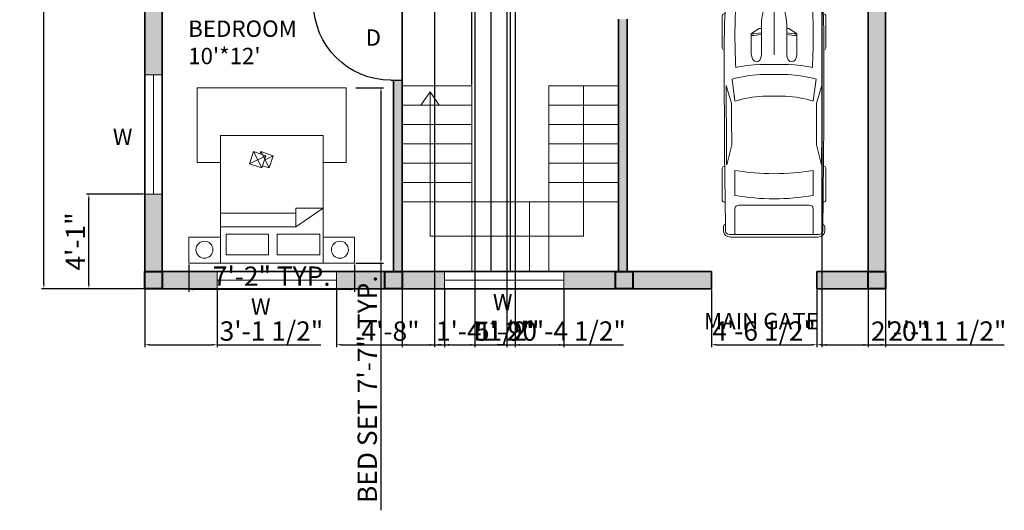
# Model space of a CAD drawing. Units: inches. Extents: x 1801 to 2333, y 2020 to 2714.
# Tile 1 of 4: x 1801 to 2311, y 2020 to 2274. Entities that reach past the tile are written whole.
import ezdxf

# ---------------------------------------------------------------- set-up
doc = ezdxf.new("R2010")
doc.units = ezdxf.units.IN
for name, color, linetype, lineweight in [('A-ANNO-DIMS', 2, 'Continuous', 18), ('A-ANNO-TEXT', 200, 'Continuous', 18), ('A-AREA-IDEN', 200, 'Continuous', 25), ('A-COLS', 7, 'Continuous', 40), ('A-COLS-PATT', 250, 'Continuous', 13), ('A-DOOR', 4, 'Continuous', 25), ('A-FLOR-STRS', 7, 'Continuous', 18), ('A-FURN', 8, 'Continuous', 18), ('A-SITE-VEHI', 8, 'Continuous', 13), ('A-WALL-PATT', 252, 'Continuous', 13), ('WALL', 150, 'Continuous', 35), ('WINDOW', 130, 'Continuous', 18)]:
    doc.layers.add(name, color=color, linetype=linetype, lineweight=lineweight)
doc.styles.get("Standard").update_dxf_attribs({"font": 'arial.ttf'})
doc.dimstyles.new('ISO-25', dxfattribs={"dimtxt": 10, "dimasz": 2.5, "dimexe": 1.25, "dimexo": 0.625, "dimtad": 1, "dimdec": 0, "dimlunit": 4, "dimtxsty": 'Standard', "dimcen": 2.5, "dimadec": 0, "dimazin": 0, "dimtfac": 1, "dimtdec": 0, "dimtmove": 0, "dimatfit": 3, "dimfxl": 1, "dimarcsym": 0})

# ---------------------------------------------------------------- blocks, each defined once
blk = doc.blocks.new('*U2')
for p, q in [((0, 0), (0, -6)), ((40, 0), (40, -6))]:
    blk.add_line(p, q)
blk.add_lwpolyline([(0, 0), (0, 40), (1.75, 40), (1.75, 0)], close=True)
blk.add_arc((0, 0), 40, 0, 90)
blk = doc.blocks.new('*U6')
for p, q in [((21.1, 37.41), (21.1, 36.83)), ((46.55, 38.89), (22.35, 38.89)), ((47.8, 37.39), (47.8, 37.41)), ((135.45, 37.07), (135.45, 37.41)), ((136.7, 38.89), (160.9, 38.89)), ((162.15, 37.41), (162.15, 36.77)), ((70.03, 31.54), (86.41, 29.35)), ((87.99, 31.87), (74.76, 35.92)), ((134.31, 35.6), (119.29, 31.78)), ((186.47, -33.5), (186.47, 33.5)), ((188.4, -32.76), (188.4, 32.76)), ((138.42, 29.35), (157.25, 29.35)), ((164.52, 26.39), (164.52, -26.39)), ((186.47, 29.35), (167.01, 29.35)), ((32.27, 11.63), (36.13, 17.17)), ((36.13, 17.17), (50.94, 17.17)), ((29.77, 9.51), (51.68, 9.51)), ((32.12, 9.51), (32.12, 11.15)), ((58.92, -10.77), (58.92, 10.77)), ((66.55, -10.53), (66.55, 10.53)), ((82.74, 8.5), (82.74, -8.5)), ((186.47, -10.53), (186.47, 10.53)), ((3.27, 6.13), (0.1, 0.41)), ((0, 0), (51.68, 0)), ((0.1, -0.41), (3.27, -6.13)), ((29.77, -9.51), (51.68, -9.51)), ((32.12, -9.51), (32.12, -11.15)), ((32.27, -11.63), (36.13, -17.17)), ((36.13, -17.17), (50.94, -17.17)), ((86.41, -29.35), (70.03, -31.54)), ((157.25, -29.35), (138.42, -29.35)), ((167.01, -29.35), (186.47, -29.35)), ((21.1, -37.41), (21.1, -36.83)), ((87.99, -31.87), (74.76, -35.92)), ((134.31, -35.6), (119.29, -31.78)), ((162.15, -37.41), (162.15, -36.77)), ((46.55, -38.89), (22.35, -38.89)), ((47.8, -37.39), (47.8, -37.41)), ((135.45, -37.07), (135.45, -37.41)), ((136.7, -38.89), (160.9, -38.89))]:
    blk.add_line(p, q)
for centre, major_axis, ratio, start_param, end_param in [((41.19, -490.86), (0, 528.23), 0.842304, 0.00281, 0.075598), ((22.35, 37.41), (0, -1.48), 0.842304, 3.141593, 4.712389), ((64.48, -10555.62), (0, 10593.03), 0.842304, -0.013397, 0.002797), ((46.55, 37.41), (0, 1.48), 0.842304, -1.570796, 0), ((136.7, 37.41), (0, -1.48), 0.842304, 3.141593, 4.712389), ((160.9, 37.41), (0, 1.48), 0.842304, -1.570796, 0), ((180.63, 35.84), (0, 2.22), 0.842304, -0.013017, 1.249894), ((64.48, -10556.36), (0, 10595.31), 0.842304, -0.013397, -0.013017), ((183.98, 32.76), (0, -5.25), 0.842304, 1.570796, 3.128196), ((266.03, -27.52), (0, 313.31), 0.842304, 1.367076, 1.39176), ((37.47, -593.96), (0, -623.33), 0.842304, 3.096046, 3.200911), ((135.29, 5.39), (0, 81.77), 0.842304, 1.245306, 1.50788), ((64.48, -10555.62), (0, -10591.55), 0.842304, 3.133765, 3.140441), ((95.79, -3666.35), (0, -3698.24), 0.842304, 3.134049, 3.144098), ((183.98, 33.5), (0, -2.96), 0.842304, 1.570796, 3.128196), ((259.18, -27.52), (0, -305.3), 0.842304, 4.528606, 4.561838), ((134.4, 5.39), (0, -89.78), 0.842304, 4.449482, 4.652344), ((149.6, 2.8), (0, -79.58), 0.842304, 4.372215, 4.640744), ((17.08, 0), (0, 147.02), 0.842304, 4.511394, 4.913384), ((35.91, 0), (0, 147.02), 0.842304, 4.511394, 4.913384), ((167.01, 26.39), (0, 2.96), 0.842304, 0, 1.570796), ((-204.49, 52.4), (0, -250.96), 0.842304, 1.385369, 1.434372), ((13.04, 17.01), (0, 27.42), 0.842304, 4.435146, 4.718221), ((14.2, 17.01), (0, 27.42), 0.842304, 4.435146, 4.718221), ((50.79, 13.34), (6.34, -0.36), 0.603834, -1.395552, 1.581315), ((29.77, -46.66), (0, 56.17), 0.842304, 0, 0.590319), ((32.75, 11.15), (0, 0.74), 0.842304, 0.879714, 1.570796), ((0.62, 0), (0, -0.74), 0.842304, 4.131459, 5.293319), ((-204.49, -52.4), (0, 250.96), 0.842304, -1.434372, -1.385369), ((29.77, 46.66), (0, 56.17), 0.842304, 2.551274, 3.141593), ((32.75, -11.15), (0, -0.74), 0.842304, 4.712389, 5.403472), ((13.04, -17.01), (0, -27.42), 0.842304, 1.564964, 1.848039), ((14.2, -17.01), (0, -27.42), 0.842304, 1.564964, 1.848039), ((134.4, -5.39), (0, -89.78), 0.842304, -1.510751, -1.307889), ((135.29, -5.39), (0, -81.77), 0.842304, -1.50788, -1.245306), ((149.6, -2.8), (0, -79.58), 0.842304, -1.499151, -1.230623), ((259.18, 27.52), (0, 305.3), 0.842304, 1.721348, 1.754579), ((266.03, 27.52), (0, 313.31), 0.842304, 1.749832, 1.774517), ((37.47, 593.96), (0, -623.33), 0.842304, -0.059319, 0.045547), ((167.01, -26.39), (0, -2.96), 0.842304, 4.712389, 6.283185), ((41.19, 490.86), (0, -528.23), 0.842304, -0.075598, -0.00281), ((64.48, 10555.62), (0, 10593.03), 0.842304, 3.138796, 3.15499), ((64.48, 10555.62), (0, -10591.55), 0.842304, 0.001152, 0.007828), ((95.79, 3666.35), (0, -3698.24), 0.842304, -0.002505, 0.007544), ((180.63, -35.84), (0, -2.22), 0.842304, -1.249894, 0.013017), ((183.98, -33.5), (0, 2.96), 0.842304, 3.15499, 4.712389), ((183.98, -32.76), (0, -5.25), 0.842304, 0.013397, 1.570796), ((22.35, -37.41), (0, 1.48), 0.842304, 1.570796, 3.141593), ((46.55, -37.41), (0, -1.48), 0.842304, 0, 1.570796), ((136.7, -37.41), (0, -1.48), 0.842304, -1.570796, 0), ((160.9, -37.41), (0, 1.48), 0.842304, 3.141593, 4.712389), ((64.48, 10556.36), (0, 10595.31), 0.842304, 3.15461, 3.15499)]:
    blk.add_ellipse(centre, major_axis=major_axis, ratio=ratio, start_param=start_param, end_param=end_param)
at = {"extrusion": (0, 0, -1)}
blk.add_ellipse((50.79, -13.34), major_axis=(6.34, 0.36), ratio=0.603834, start_param=-1.395552, end_param=1.581315, dxfattribs=at)
blk = doc.blocks.new('*D8')
at = {"layer": 'A-ANNO-DIMS', "color": 0, "lineweight": -2, "transparency": 16777216}
for p, q in [((1865.06, 2614.35), (1812.13, 2614.35)), ((1813.38, 2136.85), (1813.38, 2611.85)), ((1865.06, 2134.35), (1812.13, 2134.35))]:
    blk.add_line(p, q, dxfattribs=at)
at = {"layer": 'A-ANNO-DIMS', "color": 0, "transparency": 16777216}
for points in [[(1812.96, 2611.85), (1813.79, 2611.85), (1813.38, 2614.35)], [(1812.96, 2136.85), (1813.79, 2136.85), (1813.38, 2134.35)]]:
    blk.add_solid(points, dxfattribs=at)
at = {"layer": 'Defpoints', "color": 0, "transparency": 16777216}
for p in [(1813.38, 2614.35), (1865.69, 2614.35), (1865.69, 2134.35)]:
    blk.add_point(p, dxfattribs=at)
at = {"layer": 'A-ANNO-DIMS', "color": 0, "transparency": 16777216, "insert": (1807.65, 2374.35), "char_height": 10, "attachment_point": 5, "rotation": 90}
blk.add_mtext("40'", dxfattribs=at)
blk = doc.blocks.new('BED-DOUBLE-WITH-NIGHTSTANDS')
for p, q in [((30.54, 72.05), (16.34, 62.37)), ((69.61, 72.05), (30.54, 72.05)), ((30.54, 62.37), (30.54, 72.05)), ((16.34, 62.37), (30.54, 62.37)), ((30.54, 64.89), (69.61, 64.89)), ((44.26, 41.5), (48.62, 33.08)), ((48.1, 41.5), (52.46, 33.08)), ((16.34, 38.79), (4.34, 38.79)), ((4.34, 38.79), (4.34, 0)), ((42.19, 35.19), (46.77, 37.46)), ((46.03, 35.19), (54.53, 39.39)), ((69.61, 38.79), (81.61, 38.79)), ((81.61, 38.79), (81.61, 0)), ((4.34, 0), (81.61, 0))]:
    blk.add_line(p, q)
for points in [[(0, 90.88), (16.34, 90.88), (16.34, 77.31), (0, 77.31)], [(16.34, 90.88), (69.61, 90.88), (69.61, 24.72), (16.34, 24.72)], [(69.61, 90.88), (85.96, 90.88), (85.96, 77.31), (69.61, 77.31)], [(18.06, 86.51), (40.1, 86.51), (40.1, 75.9), (18.06, 75.9)], [(44.61, 86.51), (66.65, 86.51), (66.65, 75.9), (44.61, 75.9)], [(46.03, 35.19), (48.1, 41.5), (54.53, 39.39), (52.46, 33.08)]]:
    blk.add_lwpolyline(points, close=True)
blk.add_lwpolyline([(48.99, 34.22), (48.62, 33.08), (42.19, 35.19), (44.26, 41.5), (47.73, 40.36)])
for centre in [(7.61, 83.86), (77.85, 83.86)]:
    blk.add_circle(centre, 4.4)
blk = doc.blocks.new('WIN-STANDARD')
blk.add_line((0, 4.5), (61.87, 4.5))
blk.add_lwpolyline([(0, 9), (61.87, 9), (61.87, 0), (0, 0)], close=True)
blk = doc.blocks.new('COLUMN-9X9')
blk.add_lwpolyline([(0, 9), (9, 9), (9, 0), (0, 0)], close=True)
blk = doc.blocks.new('*D22')
at = {"layer": 'A-ANNO-DIMS', "color": 0, "lineweight": -2, "transparency": 16777216}
for p, q in [((1975.09, 2238.43), (1989.35, 2238.43)), ((1988.1, 2235.93), (1988.1, 2150.05)), ((1975.09, 2147.55), (1989.35, 2147.55)), ((1988.1, 2147.55), (1988.1, 2019.63))]:
    blk.add_line(p, q, dxfattribs=at)
at = {"layer": 'A-ANNO-DIMS', "color": 0, "transparency": 16777216}
for points in [[(1987.68, 2235.93), (1988.52, 2235.93), (1988.1, 2238.43)], [(1987.68, 2150.05), (1988.52, 2150.05), (1988.1, 2147.55)]]:
    blk.add_solid(points, dxfattribs=at)
at = {"layer": 'Defpoints', "color": 0, "transparency": 16777216}
for p in [(1974.47, 2238.43), (1974.47, 2147.55), (1988.1, 2147.55)]:
    blk.add_point(p, dxfattribs=at)
at = {"layer": 'A-ANNO-DIMS', "color": 0, "transparency": 16777216, "insert": (1982.31, 2082.34), "char_height": 10, "attachment_point": 5, "rotation": 90}
blk.add_mtext('BED SET 7\'-7" TYP.', dxfattribs=at)
blk = doc.blocks.new('*D23')
at = {"layer": 'A-ANNO-DIMS', "color": 0, "lineweight": -2, "transparency": 16777216}
for p, q in [((1888.51, 2146.93), (1888.51, 2132.67)), ((1974.47, 2146.93), (1974.47, 2132.67)), ((1971.97, 2133.92), (1891.01, 2133.92))]:
    blk.add_line(p, q, dxfattribs=at)
at = {"layer": 'A-ANNO-DIMS', "color": 0, "transparency": 16777216}
for points in [[(1891.01, 2134.34), (1891.01, 2133.5), (1888.51, 2133.92)], [(1971.97, 2134.34), (1971.97, 2133.5), (1974.47, 2133.92)]]:
    blk.add_solid(points, dxfattribs=at)
at = {"layer": 'Defpoints', "color": 0, "transparency": 16777216}
for p in [(1888.51, 2147.55), (1974.47, 2147.55), (1888.51, 2133.92)]:
    blk.add_point(p, dxfattribs=at)
at = {"layer": 'A-ANNO-DIMS', "color": 0, "transparency": 16777216, "insert": (1931.49, 2139.57), "char_height": 10, "attachment_point": 5}
blk.add_mtext('7\'-2" TYP.', dxfattribs=at)
blk = doc.blocks.new('*D36')
at = {"layer": 'A-ANNO-DIMS', "color": 0, "lineweight": -2, "transparency": 16777216}
for p, q in [((1865.06, 2183.28), (1835.44, 2183.28)), ((1836.69, 2136.85), (1836.69, 2180.78)), ((1865.06, 2134.35), (1835.44, 2134.35))]:
    blk.add_line(p, q, dxfattribs=at)
at = {"layer": 'A-ANNO-DIMS', "color": 0, "transparency": 16777216}
for points in [[(1836.27, 2180.78), (1837.11, 2180.78), (1836.69, 2183.28)], [(1836.27, 2136.85), (1837.11, 2136.85), (1836.69, 2134.35)]]:
    blk.add_solid(points, dxfattribs=at)
at = {"layer": 'Defpoints', "color": 0, "transparency": 16777216}
for p in [(1836.69, 2183.28), (1865.69, 2183.28), (1865.69, 2134.35)]:
    blk.add_point(p, dxfattribs=at)
at = {"layer": 'A-ANNO-DIMS', "color": 0, "transparency": 16777216, "insert": (1831.04, 2158.81), "char_height": 10, "attachment_point": 5, "rotation": 90}
blk.add_mtext('4\'-1"', dxfattribs=at)
blk = doc.blocks.new('*D39')
at = {"layer": 'A-ANNO-DIMS', "color": 0, "lineweight": -2, "transparency": 16777216}
for p, q in [((1865.69, 2133.72), (1865.69, 2104.1)), ((1903.28, 2133.72), (1903.28, 2104.1)), ((1868.19, 2105.35), (1900.78, 2105.35)), ((1903.28, 2105.35), (1956.91, 2105.35))]:
    blk.add_line(p, q, dxfattribs=at)
at = {"layer": 'A-ANNO-DIMS', "color": 0, "transparency": 16777216}
for points in [[(1868.19, 2105.76), (1868.19, 2104.93), (1865.69, 2105.35)], [(1900.78, 2105.76), (1900.78, 2104.93), (1903.28, 2105.35)]]:
    blk.add_solid(points, dxfattribs=at)
at = {"layer": 'Defpoints', "color": 0, "transparency": 16777216}
for p in [(1865.69, 2134.35), (1903.28, 2134.35), (1903.28, 2105.35)]:
    blk.add_point(p, dxfattribs=at)
at = {"layer": 'A-ANNO-DIMS', "color": 0, "transparency": 16777216, "insert": (1931.35, 2111.15), "char_height": 10, "attachment_point": 5}
blk.add_mtext('3\'-1 1/2"', dxfattribs=at)
blk = doc.blocks.new('*D40')
at = {"layer": 'A-ANNO-DIMS', "color": 0, "lineweight": -2, "transparency": 16777216}
for p, q in [((1965.15, 2133.72), (1965.15, 2104.1)), ((2021.01, 2133.72), (2021.01, 2104.1)), ((1967.65, 2105.35), (2018.51, 2105.35))]:
    blk.add_line(p, q, dxfattribs=at)
at = {"layer": 'A-ANNO-DIMS', "color": 0, "transparency": 16777216}
for points in [[(1967.65, 2105.76), (1967.65, 2104.93), (1965.15, 2105.35)], [(2018.51, 2105.76), (2018.51, 2104.93), (2021.01, 2105.35)]]:
    blk.add_solid(points, dxfattribs=at)
at = {"layer": 'Defpoints', "color": 0, "transparency": 16777216}
for p in [(1965.15, 2134.35), (2021.01, 2134.35), (2021.01, 2105.35)]:
    blk.add_point(p, dxfattribs=at)
at = {"layer": 'A-ANNO-DIMS', "color": 0, "transparency": 16777216, "insert": (1993.08, 2111.08), "char_height": 10, "attachment_point": 5}
blk.add_mtext('4\'-8"', dxfattribs=at)
blk = doc.blocks.new('*D41')
at = {"layer": 'A-ANNO-DIMS', "color": 0, "lineweight": -2, "transparency": 16777216}
for p, q in [((2021.01, 2133.72), (2021.01, 2104.1)), ((2082.87, 2133.72), (2082.87, 2104.1)), ((2023.51, 2105.35), (2080.37, 2105.35))]:
    blk.add_line(p, q, dxfattribs=at)
at = {"layer": 'A-ANNO-DIMS', "color": 0, "transparency": 16777216}
for points in [[(2023.51, 2105.76), (2023.51, 2104.93), (2021.01, 2105.35)], [(2080.37, 2105.76), (2080.37, 2104.93), (2082.87, 2105.35)]]:
    blk.add_solid(points, dxfattribs=at)
at = {"layer": 'Defpoints', "color": 0, "transparency": 16777216}
for p in [(2021.01, 2134.35), (2082.87, 2134.35), (2082.87, 2105.35)]:
    blk.add_point(p, dxfattribs=at)
at = {"layer": 'A-ANNO-DIMS', "color": 0, "transparency": 16777216, "insert": (2051.94, 2111.08), "char_height": 10, "attachment_point": 5}
blk.add_mtext('5\'-2"', dxfattribs=at)
blk = doc.blocks.new('*D42')
at = {"layer": 'A-ANNO-DIMS', "color": 0, "lineweight": -2, "transparency": 16777216}
for p, q in [((2159.47, 2133.72), (2159.47, 2104.1)), ((2214.05, 2133.72), (2214.05, 2104.1)), ((2161.97, 2105.35), (2211.55, 2105.35))]:
    blk.add_line(p, q, dxfattribs=at)
at = {"layer": 'A-ANNO-DIMS', "color": 0, "transparency": 16777216}
for points in [[(2161.97, 2105.76), (2161.97, 2104.93), (2159.47, 2105.35)], [(2211.55, 2105.76), (2211.55, 2104.93), (2214.05, 2105.35)]]:
    blk.add_solid(points, dxfattribs=at)
at = {"layer": 'Defpoints', "color": 0, "transparency": 16777216}
for p in [(2159.47, 2134.35), (2214.05, 2134.35), (2214.05, 2105.35)]:
    blk.add_point(p, dxfattribs=at)
at = {"layer": 'A-ANNO-DIMS', "color": 0, "transparency": 16777216, "insert": (2186.76, 2111.14), "char_height": 10, "attachment_point": 5}
blk.add_mtext('4\'-6 1/2"', dxfattribs=at)
blk = doc.blocks.new('*D43')
at = {"layer": 'A-ANNO-DIMS', "color": 0, "lineweight": -2, "transparency": 16777216}
for p, q in [((2214.05, 2133.72), (2214.05, 2104.1)), ((2249.69, 2133.72), (2249.69, 2104.1)), ((2216.55, 2105.35), (2247.19, 2105.35)), ((2249.69, 2105.35), (2311.26, 2105.35))]:
    blk.add_line(p, q, dxfattribs=at)
at = {"layer": 'A-ANNO-DIMS', "color": 0, "transparency": 16777216}
for points in [[(2216.55, 2105.76), (2216.55, 2104.93), (2214.05, 2105.35)], [(2247.19, 2105.76), (2247.19, 2104.93), (2249.69, 2105.35)]]:
    blk.add_solid(points, dxfattribs=at)
at = {"layer": 'Defpoints', "color": 0, "transparency": 16777216}
for p in [(2214.05, 2134.35), (2249.69, 2134.35), (2249.69, 2105.35)]:
    blk.add_point(p, dxfattribs=at)
at = {"layer": 'A-ANNO-DIMS', "color": 0, "transparency": 16777216, "insert": (2281.73, 2111.14), "char_height": 10, "attachment_point": 5}
blk.add_mtext('2\'-11 1/2"', dxfattribs=at)
blk = doc.blocks.new('*D44')
at = {"layer": 'A-ANNO-DIMS', "color": 0, "lineweight": -2, "transparency": 16777216}
for p, q in [((1999.19, 2239.97), (1999.19, 2694.33)), ((2001.69, 2693.08), (2032.69, 2693.08)), ((2035.19, 2239.97), (2035.19, 2694.33))]:
    blk.add_line(p, q, dxfattribs=at)
at = {"layer": 'A-ANNO-DIMS', "color": 0, "transparency": 16777216}
for points in [[(2001.69, 2693.5), (2001.69, 2692.66), (1999.19, 2693.08)], [(2032.69, 2693.5), (2032.69, 2692.66), (2035.19, 2693.08)]]:
    blk.add_solid(points, dxfattribs=at)
at = {"layer": 'Defpoints', "color": 0, "transparency": 16777216}
for p in [(2035.19, 2693.08), (1999.19, 2239.35), (2035.19, 2239.35)]:
    blk.add_point(p, dxfattribs=at)
at = {"layer": 'A-ANNO-DIMS', "color": 0, "transparency": 16777216, "insert": (2017.19, 2698.81), "char_height": 10, "attachment_point": 5}
blk.add_mtext('3\'-0"', dxfattribs=at)
blk = doc.blocks.new('*D45')
at = {"layer": 'A-ANNO-DIMS', "color": 0, "lineweight": -2, "transparency": 16777216}
for p, q in [((2045.19, 2143.97), (2045.19, 2694.33)), ((2047.69, 2693.08), (2052.69, 2693.08)), ((2055.19, 2143.97), (2055.19, 2694.33)), ((2055.19, 2693.08), (2093.29, 2693.08))]:
    blk.add_line(p, q, dxfattribs=at)
at = {"layer": 'A-ANNO-DIMS', "color": 0, "transparency": 16777216}
for points in [[(2047.69, 2693.5), (2047.69, 2692.66), (2045.19, 2693.08)], [(2052.69, 2693.5), (2052.69, 2692.66), (2055.19, 2693.08)]]:
    blk.add_solid(points, dxfattribs=at)
at = {"layer": 'Defpoints', "color": 0, "transparency": 16777216}
for p in [(2055.19, 2693.08), (2045.19, 2143.35), (2055.19, 2143.35)]:
    blk.add_point(p, dxfattribs=at)
at = {"layer": 'A-ANNO-DIMS', "color": 0, "transparency": 16777216, "insert": (2075.49, 2698.81), "char_height": 10, "attachment_point": 5}
blk.add_mtext('0\'-10"', dxfattribs=at)
blk = doc.blocks.new('*D46')
at = {"layer": 'A-ANNO-DIMS', "color": 0, "lineweight": -2, "transparency": 16777216}
for p, q in [((2216.69, 2444.22), (2216.69, 2104.1)), ((2240.69, 2444.22), (2240.69, 2104.1)), ((2219.19, 2105.35), (2238.19, 2105.35)), ((2240.69, 2105.35), (2271.19, 2105.35))]:
    blk.add_line(p, q, dxfattribs=at)
at = {"layer": 'A-ANNO-DIMS', "color": 0, "transparency": 16777216}
for points in [[(2219.19, 2105.76), (2219.19, 2104.93), (2216.69, 2105.35)], [(2238.19, 2105.76), (2238.19, 2104.93), (2240.69, 2105.35)]]:
    blk.add_solid(points, dxfattribs=at)
at = {"layer": 'Defpoints', "color": 0, "transparency": 16777216}
for p in [(2216.69, 2444.85), (2240.69, 2444.85), (2240.69, 2105.35)]:
    blk.add_point(p, dxfattribs=at)
at = {"layer": 'A-ANNO-DIMS', "color": 0, "transparency": 16777216, "insert": (2257.19, 2111.08), "char_height": 10, "attachment_point": 5}
blk.add_mtext('2\'-0"', dxfattribs=at)
blk = doc.blocks.new('*D47')
at = {"layer": 'A-ANNO-DIMS', "color": 0, "lineweight": -2, "transparency": 16777216}
for p, q in [((2053.36, 2604.46), (2053.36, 2104.1)), ((2057.69, 2604.72), (2057.69, 2104.1)), ((2050.86, 2105.35), (2048.36, 2105.35)), ((2053.36, 2105.35), (2057.69, 2105.35)), ((2060.19, 2105.35), (2113.82, 2105.35))]:
    blk.add_line(p, q, dxfattribs=at)
at = {"layer": 'A-ANNO-DIMS', "color": 0, "transparency": 16777216}
for points in [[(2050.86, 2105.76), (2050.86, 2104.93), (2053.36, 2105.35)], [(2060.19, 2105.76), (2060.19, 2104.93), (2057.69, 2105.35)]]:
    blk.add_solid(points, dxfattribs=at)
at = {"layer": 'Defpoints', "color": 0, "transparency": 16777216}
for p in [(2053.36, 2605.08), (2057.69, 2605.35), (2057.69, 2105.35)]:
    blk.add_point(p, dxfattribs=at)
at = {"layer": 'A-ANNO-DIMS', "color": 0, "transparency": 16777216, "insert": (2088.26, 2111.14), "char_height": 10, "attachment_point": 5}
blk.add_mtext('0\'-4 1/2"', dxfattribs=at)
blk = doc.blocks.new('*D55')
at = {"layer": 'A-ANNO-DIMS', "color": 0, "lineweight": -2, "transparency": 16777216}
for p, q in [((1999.19, 2604.72), (1999.19, 2104.1)), ((2015.86, 2603.46), (2015.86, 2104.1)), ((2001.69, 2105.35), (2013.36, 2105.35)), ((2015.86, 2105.35), (2068.55, 2105.35))]:
    blk.add_line(p, q, dxfattribs=at)
at = {"layer": 'A-ANNO-DIMS', "color": 0, "transparency": 16777216}
for points in [[(2001.69, 2105.76), (2001.69, 2104.93), (1999.19, 2105.35)], [(2013.36, 2105.76), (2013.36, 2104.93), (2015.86, 2105.35)]]:
    blk.add_solid(points, dxfattribs=at)
at = {"layer": 'Defpoints', "color": 0, "transparency": 16777216}
for p in [(1999.19, 2605.35), (2015.86, 2604.08), (2015.86, 2105.35)]:
    blk.add_point(p, dxfattribs=at)
at = {"layer": 'A-ANNO-DIMS', "color": 0, "transparency": 16777216, "insert": (2043.46, 2111.14), "char_height": 10, "attachment_point": 5}
blk.add_mtext('1\'-4 1/2"', dxfattribs=at)
blk = doc.blocks.new('*D56')
at = {"layer": 'A-ANNO-DIMS', "color": 0, "lineweight": -2, "transparency": 16777216}
for p, q in [((2015.86, 2603.46), (2015.86, 2104.1)), ((2036.86, 2603.46), (2036.86, 2104.1)), ((2018.36, 2105.35), (2034.36, 2105.35)), ((2036.86, 2105.35), (2066.25, 2105.35))]:
    blk.add_line(p, q, dxfattribs=at)
at = {"layer": 'A-ANNO-DIMS', "color": 0, "transparency": 16777216}
for points in [[(2018.36, 2105.76), (2018.36, 2104.93), (2015.86, 2105.35)], [(2034.36, 2105.76), (2034.36, 2104.93), (2036.86, 2105.35)]]:
    blk.add_solid(points, dxfattribs=at)
at = {"layer": 'Defpoints', "color": 0, "transparency": 16777216}
for p in [(2015.86, 2604.08), (2036.86, 2604.08), (2036.86, 2105.35)]:
    blk.add_point(p, dxfattribs=at)
at = {"layer": 'A-ANNO-DIMS', "color": 0, "transparency": 16777216, "insert": (2052.81, 2111.08), "char_height": 10, "attachment_point": 5}
blk.add_mtext('1\'-9"', dxfattribs=at)

msp = doc.modelspace()

# ---------------------------------------------------------------- hatches: boundary and pattern name
at = {"layer": 'A-COLS-PATT'}
h = msp.add_hatch(color=256, dxfattribs=at)
h.dxf.hatch_style = 1
h.paths.add_polyline_path([(1874.69, 2614.35), (1865.69, 2614.35), (1865.69, 2605.35), (1874.69, 2605.35)])
h.paths.add_polyline_path([(2002.83, 2614.35), (1993.83, 2614.35), (1993.83, 2605.35), (2002.83, 2605.35)])
h.paths.add_polyline_path([(2117.06, 2614.35), (2108.06, 2614.35), (2108.06, 2605.35), (2117.06, 2605.35)])
h.paths.add_polyline_path([(2249.69, 2614.35), (2240.69, 2614.35), (2240.69, 2605.35), (2249.69, 2605.35)])
h.paths.add_polyline_path([(1874.69, 2452.27), (1865.69, 2452.27), (1865.69, 2443.27), (1874.69, 2443.27)])
h.paths.add_polyline_path([(1999.19, 2449.12), (1990.19, 2449.12), (1990.19, 2444.85), (1999.19, 2444.85)])
h.paths.add_polyline_path([(1999.19, 2444.85), (1990.19, 2444.85), (1990.19, 2440.12), (1999.19, 2440.12)])
h.paths.add_polyline_path([(2120.9, 2449.35), (2116.19, 2449.35), (2116.19, 2453.56), (2111.9, 2453.56), (2111.9, 2444.85), (2120.9, 2444.85)])
h.paths.add_polyline_path([(2120.9, 2453.56), (2116.19, 2453.56), (2116.19, 2449.35), (2120.9, 2449.35)], flags=17)
h.paths.add_polyline_path([(2249.69, 2451.04), (2240.69, 2451.04), (2240.69, 2442.04), (2249.69, 2442.04)])
h.paths.add_polyline_path([(2249.69, 2330.92), (2240.69, 2330.92), (2240.69, 2321.92), (2249.69, 2321.92)])
h.paths.add_polyline_path([(2115.69, 2329.7), (2111.19, 2329.7), (2111.19, 2324.35), (2115.69, 2324.35)])
h.paths.add_polyline_path([(2115.69, 2324.35), (2111.19, 2324.35), (2111.19, 2320.7), (2115.69, 2320.7)])
h.paths.add_polyline_path([(2111.19, 2329.7), (2106.69, 2329.7), (2106.69, 2320.7), (2111.19, 2320.7), (2111.19, 2324.35)])
h.paths.add_polyline_path([(1999.19, 2291.85), (1991.86, 2291.85), (1991.86, 2287.35), (1994.69, 2287.35), (1994.69, 2283.08), (1999.19, 2283.08)], flags=17)
h.paths.add_polyline_path([(2000.86, 2292.08), (1991.86, 2292.08), (1991.86, 2291.85), (1999.19, 2291.85), (1999.19, 2283.08), (2000.86, 2283.08)])
h.paths.add_polyline_path([(1994.69, 2287.35), (1991.86, 2287.35), (1991.86, 2283.08), (1994.69, 2283.08)], flags=16)
h.paths.add_polyline_path([(1874.69, 2143.35), (1865.69, 2143.35), (1865.69, 2134.35), (1874.69, 2134.35)])
h.paths.add_polyline_path([(1999.19, 2143.35), (1990.19, 2143.35), (1990.19, 2134.35), (1999.19, 2134.35)])
h.paths.add_polyline_path([(2118.63, 2143.35), (2109.63, 2143.35), (2109.63, 2134.35), (2118.63, 2134.35)])
h.paths.add_polyline_path([(2249.69, 2143.35), (2240.69, 2143.35), (2240.69, 2134.35), (2249.69, 2134.35)])
at = {"layer": 'A-WALL-PATT'}
h = msp.add_hatch(color=256, dxfattribs=at)
h.dxf.hatch_style = 1
h.paths.add_polyline_path([(2067.79, 2614.35), (2044.01, 2614.35), (2044.01, 2605.35), (2053.19, 2605.35), (2067.79, 2605.35)])
h.paths.add_polyline_path([(2057.69, 2605.35), (2053.19, 2605.35), (2053.19, 2509.35), (2040.35, 2509.35), (2030.72, 2509.35), (2030.72, 2504.85), (2040.35, 2504.85), (2057.69, 2504.85), (2111.69, 2504.85), (2111.69, 2509.35), (2057.69, 2509.35)])
h.paths.add_polyline_path([(1999.19, 2605.35), (1994.69, 2605.35), (1994.69, 2490.6), (1999.19, 2490.6)])
h.paths.add_polyline_path([(2116.19, 2605.35), (2111.69, 2605.35), (2111.69, 2550.35), (2111.69, 2535.67, -0.006913), (2112.39, 2535.68), (2116.19, 2535.68), (2116.19, 2551.5)])
h.paths.add_polyline_path([(2116.19, 2510.35), (2112.39, 2510.35), (2111.69, 2510.35), (2111.69, 2495.25), (2116.19, 2495.25)])
h.paths.add_polyline_path([(2115.69, 2273.91), (2111.19, 2273.91), (2111.19, 2143.35), (2115.69, 2143.35)], flags=17)
h.paths.add_polyline_path([(2118.63, 2143.35), (2118.63, 2134.35), (2159.47, 2134.35), (2159.47, 2143.35)])
h.paths.add_polyline_path([(2109.63, 2134.35), (2109.63, 2143.35), (2082.87, 2143.35), (2082.87, 2134.35)])
h.paths.add_polyline_path([(1999.19, 2143.35), (1999.19, 2134.35), (2021.01, 2134.35), (2021.01, 2143.35)])
h.paths.add_polyline_path([(1990.19, 2134.35), (1990.19, 2143.35), (1965.15, 2143.35), (1965.15, 2134.35)])
h.paths.add_polyline_path([(1903.28, 2143.35), (1874.69, 2143.35), (1874.69, 2134.35), (1903.28, 2134.35)])
h.paths.add_polyline_path([(1865.69, 2143.35), (1874.69, 2143.35), (1874.69, 2183.28), (1865.69, 2183.28)])
h.paths.add_polyline_path([(1991.86, 2287.35), (1991.86, 2291.85), (1874.69, 2291.85), (1874.69, 2287.35)])
h.paths.add_polyline_path([(1999.19, 2283.08), (1994.69, 2283.08), (1994.69, 2282.32), (1999.19, 2282.32)])
h.paths.add_polyline_path([(1865.69, 2452.27), (1874.69, 2452.27), (1874.69, 2515.15), (1865.69, 2515.15)])
h.paths.add_polyline_path([(1874.69, 2443.27), (1865.69, 2443.27), (1865.69, 2400.61), (1874.69, 2400.61)])
h.paths.add_polyline_path([(2120.9, 2449.35), (2120.9, 2444.85), (2240.69, 2444.85), (2240.69, 2449.35)])
h.paths.add_polyline_path([(2111.9, 2453.56), (2116.19, 2453.56), (2116.19, 2455.25), (2111.69, 2455.25), (2111.69, 2444.85), (2111.9, 2444.85)])
h.paths.add_polyline_path([(1874.69, 2605.35), (1865.69, 2605.35), (1865.69, 2577.02), (1874.69, 2577.02)])
h.paths.add_polyline_path([(1874.69, 2614.35), (1874.69, 2605.35), (1903.59, 2605.35), (1903.59, 2614.35)])
h = msp.add_hatch(color=256, dxfattribs=at)
h.dxf.hatch_style = 1
h.paths.add_polyline_path([(2118.63, 2143.35), (2118.63, 2134.35), (2159.47, 2134.35), (2159.47, 2143.35)])
h.paths.add_polyline_path([(2109.63, 2134.35), (2109.63, 2143.35), (2082.87, 2143.35), (2082.87, 2134.35)])
h.paths.add_polyline_path([(1999.19, 2143.35), (1999.19, 2134.35), (2021.01, 2134.35), (2021.01, 2143.35)])
h.paths.add_polyline_path([(1990.19, 2134.35), (1990.19, 2143.35), (1965.15, 2143.35), (1965.15, 2134.35)])
h.paths.add_polyline_path([(1874.69, 2143.35), (1874.69, 2134.35), (1903.28, 2134.35), (1903.28, 2143.35)])
h.paths.add_polyline_path([(1865.69, 2143.35), (1874.69, 2143.35), (1874.69, 2183.28), (1865.69, 2183.28)])
h.paths.add_polyline_path([(1874.69, 2443.27), (1865.69, 2443.27), (1865.69, 2400.61), (1874.69, 2400.61)])
h.paths.add_polyline_path([(1865.69, 2452.27), (1874.69, 2452.27), (1874.69, 2515.15), (1865.69, 2515.15)])
h.paths.add_polyline_path([(1874.69, 2577.02), (1874.69, 2605.35), (1865.69, 2605.35), (1865.69, 2577.02)])
h.paths.add_polyline_path([(1874.69, 2614.35), (1874.69, 2605.35), (1903.59, 2605.35), (1903.59, 2614.35)])
h.paths.add_polyline_path([(2240.69, 2605.35), (2240.69, 2614.35), (2203.01, 2614.35), (2203.01, 2605.35)])
h.paths.add_polyline_path([(2249.69, 2605.35), (2240.69, 2605.35), (2240.69, 2567.46), (2249.69, 2567.46)])
h = msp.add_hatch(color=256, dxfattribs=at)
h.dxf.hatch_style = 1
h.paths.add_polyline_path([(2249.69, 2505.59), (2240.69, 2505.59), (2240.69, 2451.04), (2249.69, 2451.04)])
h.paths.add_polyline_path([(2249.69, 2442.04), (2240.69, 2442.04), (2240.69, 2424.01), (2249.69, 2424.01)])
h.paths.add_polyline_path([(2249.69, 2362.14), (2240.69, 2362.14), (2240.69, 2330.92), (2249.69, 2330.92)])
h.paths.add_polyline_path([(2249.69, 2321.92), (2240.69, 2321.92), (2240.69, 2143.35), (2249.69, 2143.35)])
h.paths.add_polyline_path([(2240.69, 2143.35), (2214.05, 2143.35), (2214.05, 2134.35), (2240.69, 2134.35)])
h.paths.add_polyline_path([(1874.69, 2282.85), (1865.69, 2282.85), (1865.69, 2245.15), (1874.69, 2245.15)])
h.paths.add_polyline_path([(1874.69, 2338.74), (1865.69, 2338.74), (1865.69, 2291.85), (1874.69, 2291.85)])
h.paths.add_polyline_path([(1990.19, 2449.12), (1999.19, 2449.12), (1999.19, 2450.6), (1994.69, 2450.6), (1994.69, 2449.35), (1874.69, 2449.35), (1874.69, 2444.85), (1990.19, 2444.85)])
h.paths.add_polyline_path([(2141.14, 2614.35), (2117.06, 2614.35), (2117.06, 2605.35), (2141.14, 2605.35)])
h.paths.add_polyline_path([(2108.06, 2614.35), (2102.92, 2614.35), (2102.92, 2605.35), (2108.06, 2605.35)])
h.paths.add_polyline_path([(1993.83, 2614.35), (1965.46, 2614.35), (1965.46, 2605.35), (1993.83, 2605.35)])
h.paths.add_polyline_path([(2008.88, 2614.35), (2002.83, 2614.35), (2002.83, 2605.35), (2008.88, 2605.35)])
h.paths.add_polyline_path([(2107.38, 2466.24), (2120.18, 2466.24), (2120.18, 2483.72), (2107.38, 2483.72)], flags=9)
h.paths.add_polyline_path([(2104.14, 2515.21), (2116.94, 2515.21), (2116.94, 2532.69), (2104.14, 2532.69)], flags=9)
h.paths.add_polyline_path([(2007.5, 2499.97), (2020.3, 2499.97), (2020.3, 2517.44), (2007.5, 2517.44)], flags=9)
h.paths.add_polyline_path([(1985.91, 2461.68), (1998.7, 2461.68), (1998.7, 2479.15), (1985.91, 2479.15)], flags=9)
h.paths.add_polyline_path([(2109.98, 2348.28), (2122.78, 2348.28), (2122.78, 2365.76), (2109.98, 2365.76)], flags=9)
h.paths.add_polyline_path([(1977.13, 2255.51), (1989.93, 2255.51), (1989.93, 2272.99), (1977.13, 2272.99)], flags=9)
h.paths.add_polyline_path([(2063.1, 2540.71), (2101.48, 2540.71), (2101.48, 2560.24), (2063.1, 2560.24)], flags=9)
h.paths.add_polyline_path([(1995.81, 2316.5), (2071.83, 2316.5), (2071.83, 2348.15), (1995.81, 2348.15)], flags=9)
h.paths.add_polyline_path([(2138.31, 2394.68), (2194.97, 2394.68), (2194.97, 2426.33), (2138.31, 2426.33)], flags=9)
h.paths.add_polyline_path([(2163.82, 2472.81), (2229.7, 2472.81), (2229.7, 2504.45), (2163.82, 2504.45)], flags=9)
h.paths.add_polyline_path([(2007.01, 2540.94), (2045.38, 2540.94), (2045.38, 2560.47), (2007.01, 2560.47)], flags=9)
h.paths.add_polyline_path([(1882.98, 2452.95), (1948.86, 2452.95), (1948.86, 2484.59), (1882.98, 2484.59)], flags=9)
h = msp.add_hatch(color=256, dxfattribs=at)
h.dxf.hatch_style = 1
h.paths.add_polyline_path([(2115.69, 2444.85), (2111.69, 2444.85), (2111.69, 2375.54), (2115.69, 2375.54)])
h.paths.add_polyline_path([(2115.69, 2324.35), (2111.19, 2324.35), (2111.19, 2313.91), (2115.69, 2313.91)])
h.paths.add_polyline_path([(1999.19, 2242.32), (1994.69, 2242.32), (1994.69, 2143.35), (1999.19, 2143.35), (1999.19, 2179.35)])

# ---------------------------------------------------------------- linework, layer by layer
at = {"layer": 'A-FLOR-STRS'}
for p, q in [((1999.19, 2239.35), (2035.19, 2239.35)), ((2013.58, 2236.34), (2008.86, 2229.35)), ((2013.58, 2161.51), (2013.58, 2236.34)), ((2013.58, 2236.34), (2018.31, 2229.35)), ((2035.19, 2179.35), (2035.19, 2239.35)), ((2075.19, 2179.35), (2075.19, 2239.35)), ((2075.19, 2239.35), (2111.19, 2239.35)), ((2093.19, 2239.35), (2093.19, 2161.51)), ((1999.19, 2229.35), (2035.19, 2229.35)), ((2075.19, 2229.35), (2111.19, 2229.35)), ((1999.19, 2219.35), (2035.19, 2219.35)), ((2075.19, 2219.35), (2111.19, 2219.35)), ((1999.19, 2209.35), (2035.19, 2209.35)), ((2075.19, 2209.35), (2111.19, 2209.35)), ((1999.19, 2199.35), (2035.19, 2199.35)), ((2075.19, 2199.35), (2111.19, 2199.35)), ((1999.19, 2189.35), (2035.19, 2189.35)), ((2075.19, 2189.35), (2111.19, 2189.35)), ((1999.19, 2143.35), (1999.19, 2179.35)), ((2035.19, 2179.35), (1999.19, 2179.35)), ((1999.19, 2179.35), (2111.19, 2179.35)), ((2035.19, 2179.35), (2075.19, 2179.35)), ((2035.19, 2179.35), (2035.19, 2143.35)), ((2045.19, 2179.35), (2045.19, 2143.35)), ((2055.19, 2179.35), (2055.19, 2143.35)), ((2065.19, 2179.35), (2065.19, 2143.35)), ((2075.19, 2179.35), (2075.19, 2143.35)), ((2093.19, 2161.51), (2013.58, 2161.51)), ((1999.19, 2143.35), (2035.19, 2143.35)), ((2111.19, 2143.35), (2075.19, 2143.35))]:
    msp.add_line(p, q, dxfattribs=at)
at = {"layer": 'WALL'}
for p, q in [((2111.19, 2143.35), (2111.19, 2273.91)), ((2115.69, 2143.35), (2115.69, 2273.91)), ((1994.69, 2143.35), (1994.69, 2242.32)), ((1999.19, 2143.35), (1999.19, 2242.32)), ((1874.69, 2143.35), (1994.69, 2143.35)), ((2159.47, 2143.35), (2115.69, 2143.35)), ((2159.47, 2143.35), (2159.47, 2134.35)), ((2240.69, 2143.35), (2214.05, 2143.35)), ((2214.05, 2143.35), (2214.05, 2134.35))]:
    msp.add_line(p, q, dxfattribs=at)
for points in [[(2214.05, 2134.35), (2249.69, 2134.35), (2249.69, 2614.35), (1865.69, 2614.35), (1865.69, 2134.35), (2159.47, 2134.35)], [(2214.05, 2143.35), (2240.69, 2143.35), (2240.69, 2605.35), (1874.69, 2605.35), (1874.69, 2143.35), (2159.47, 2143.35)]]:
    msp.add_lwpolyline(points, dxfattribs=at)
at = {"layer": 'WINDOW'}
msp.add_line((2021.01, 2138.85), (2082.87, 2138.85), dxfattribs=at)
msp.add_lwpolyline([(2021.01, 2134.35), (2021.01, 2143.35), (2082.87, 2143.35), (2082.87, 2134.35)], dxfattribs=at)

# ---------------------------------------------------------------- block references
at = {"layer": 'A-COLS'}
for p in [(1865.69, 2134.35), (1990.19, 2134.35), (2109.63, 2134.35), (2240.69, 2134.35)]:
    msp.add_blockref('COLUMN-9X9', p, dxfattribs=at)
at = {"layer": 'A-DOOR', "xscale": -1, "rotation": 90}
msp.add_blockref('*U2', (1993.19, 2282.32), dxfattribs=at)
at = {"layer": 'A-FURN', "rotation": 180}
msp.add_blockref('BED-DOUBLE-WITH-NIGHTSTANDS', (1974.47, 2238.43), dxfattribs=at)
at = {"layer": 'A-SITE-VEHI', "xscale": 0.6906338309990653, "yscale": 0.6906338309990653, "zscale": 0.6906338309990653, "rotation": 270}
msp.add_blockref('*U6', (2191.92, 2291.24), dxfattribs=at)
at = {"layer": 'WINDOW', "rotation": 270.0000000000001}
msp.add_blockref('WIN-STANDARD', (1865.69, 2245.15), dxfattribs=at)
at = {"layer": 'WINDOW'}
msp.add_blockref('WIN-STANDARD', (1903.28, 2134.35), dxfattribs=at)

# ---------------------------------------------------------------- texts
at = {"layer": 'A-ANNO-TEXT', "attachment_point": 1}
for s, insert, char_height in [('D', (1980.17, 2268.63), 8.48), ('W', (1849.13, 2217.24), 8.48), ('W', (1920.73, 2129.34), 8.48), ('W', (2046.14, 2131.67), 8.48), ('MAIN GATE', (2155.57, 2121.84), 8.481)]:
    msp.add_mtext_dynamic_manual_height_columns(s, width=170.2706, gutter_width=42.4, heights=[0], dxfattribs=dict(at, insert=insert, char_height=char_height))
at = {"layer": 'A-AREA-IDEN', "insert": (1888.19, 2273.24), "char_height": 8.481, "attachment_point": 1}
msp.add_mtext_dynamic_manual_height_columns("BEDROOM\\P10'*12'", width=170.2706, gutter_width=42.4, heights=[0], dxfattribs=at)

# ---------------------------------------------------------------- dimensions: what is measured, and where the dimension line sits
at = {"layer": 'A-ANNO-DIMS'}
for base, p1, p2, picture, middle in [((2035.19, 2693.08), (1999.19, 2239.35), (2035.19, 2239.35), '*D44', (2017.19, 2698.81)), ((2055.19, 2693.08), (2045.19, 2143.35), (2055.19, 2143.35), '*D45', (2075.49, 2698.81)), ((2015.86, 2105.35), (1999.19, 2605.35), (2015.86, 2604.08), '*D55', (2043.46, 2111.14)), ((2036.86, 2105.35), (2015.86, 2604.08), (2036.86, 2604.08), '*D56', (2052.81, 2111.08)), ((2057.69, 2105.35), (2053.36, 2605.08), (2057.69, 2605.35), '*D47', (2088.26, 2111.14)), ((2240.69, 2105.35), (2216.69, 2444.85), (2240.69, 2444.85), '*D46', (2257.19, 2111.08)), ((1903.28, 2105.35), (1865.69, 2134.35), (1903.28, 2134.35), '*D39', (1931.35, 2111.15)), ((2021.01, 2105.35), (1965.15, 2134.35), (2021.01, 2134.35), '*D40', (1993.08, 2111.08)), ((2082.87, 2105.35), (2021.01, 2134.35), (2082.87, 2134.35), '*D41', (2051.94, 2111.08)), ((2214.05, 2105.35), (2159.47, 2134.35), (2214.05, 2134.35), '*D42', (2186.76, 2111.14)), ((2249.69, 2105.35), (2214.05, 2134.35), (2249.69, 2134.35), '*D43', (2281.73, 2111.14))]:
    dim = msp.add_linear_dim(base=base, p1=p1, p2=p2, dimstyle='ISO-25', override={"dimdec": 1, "dimlfac": 1, "dimrnd": 0, "dimzin": 1, "dimdsep": 46, "dimlunit": 4, "dimfrac": 2}, dxfattribs=at)
    dim.commit()
    dim.dimension.update_dxf_attribs({"geometry": picture, "text_midpoint": middle})
for base, p2, override, picture, middle in [((1813.38, 2614.35), (1865.69, 2614.35), {"dimclrd": 0, "dimclre": 0, "dimclrt": 0}, '*D8', (1807.65, 2374.35)), ((1836.69, 2183.28), (1865.69, 2183.28), {"dimdec": 1, "dimlfac": 1, "dimrnd": 0, "dimzin": 1, "dimdsep": 46, "dimlunit": 4, "dimfrac": 2}, '*D36', (1831.04, 2158.81))]:
    dim = msp.add_linear_dim(base=base, p1=(1865.69, 2134.35), p2=p2, angle=90, dimstyle='ISO-25', override=override, dxfattribs=at)
    dim.commit()
    dim.dimension.update_dxf_attribs({"geometry": picture, "text_midpoint": middle})
for base, p1, p2, angle, text, picture, middle in [((1988.1, 2147.55), (1974.47, 2238.43), (1974.47, 2147.55), 270, 'BED SET <> TYP.', '*D22', (1982.31, 2082.34)), ((1888.51, 2133.92), (1974.47, 2147.55), (1888.51, 2147.55), 180, '<> TYP.', '*D23', (1931.49, 2139.57))]:
    dim = msp.add_linear_dim(base=base, p1=p1, p2=p2, angle=angle, text=text, dimstyle='ISO-25', override={"dimdec": 1, "dimlfac": 1, "dimrnd": 0, "dimzin": 1, "dimdsep": 46, "dimlunit": 4, "dimfrac": 2}, dxfattribs=at)
    dim.commit()
    dim.dimension.update_dxf_attribs({"geometry": picture, "text_midpoint": middle})

doc.saveas('drawing.dxf')
